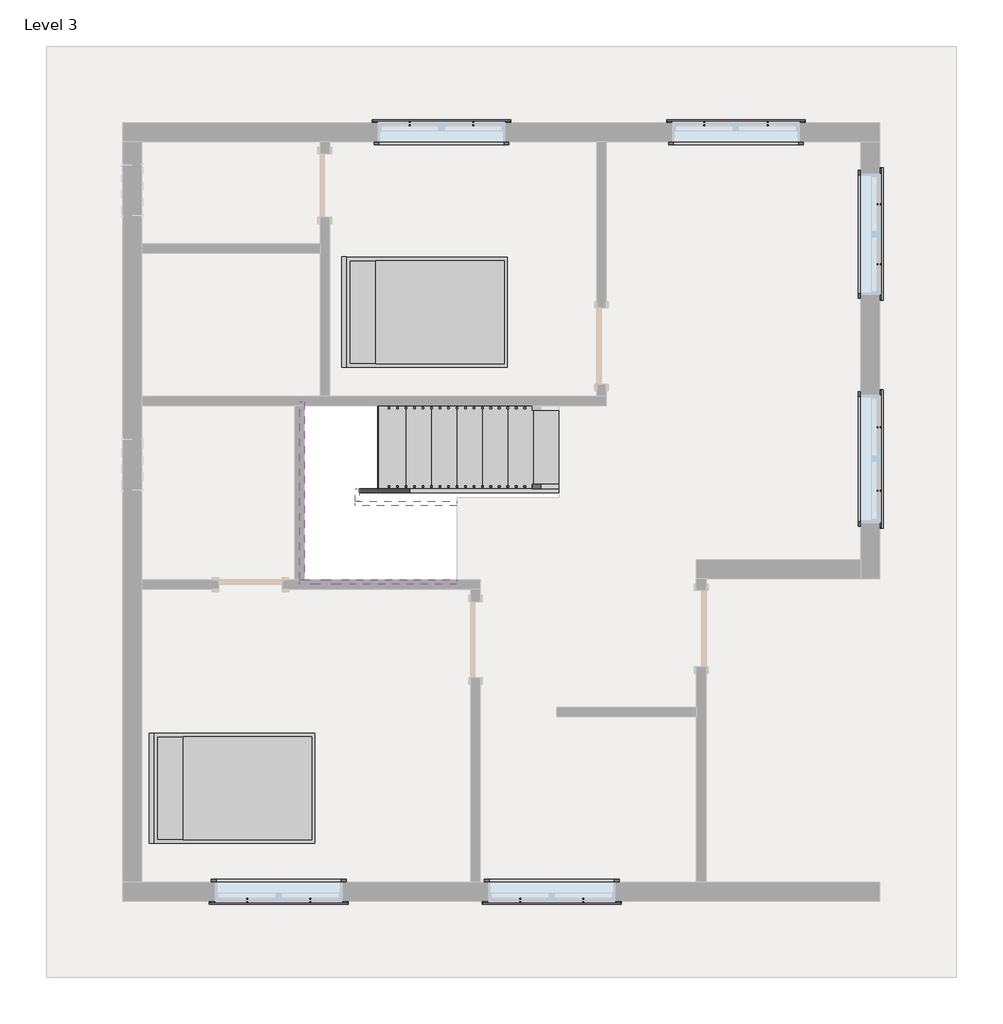
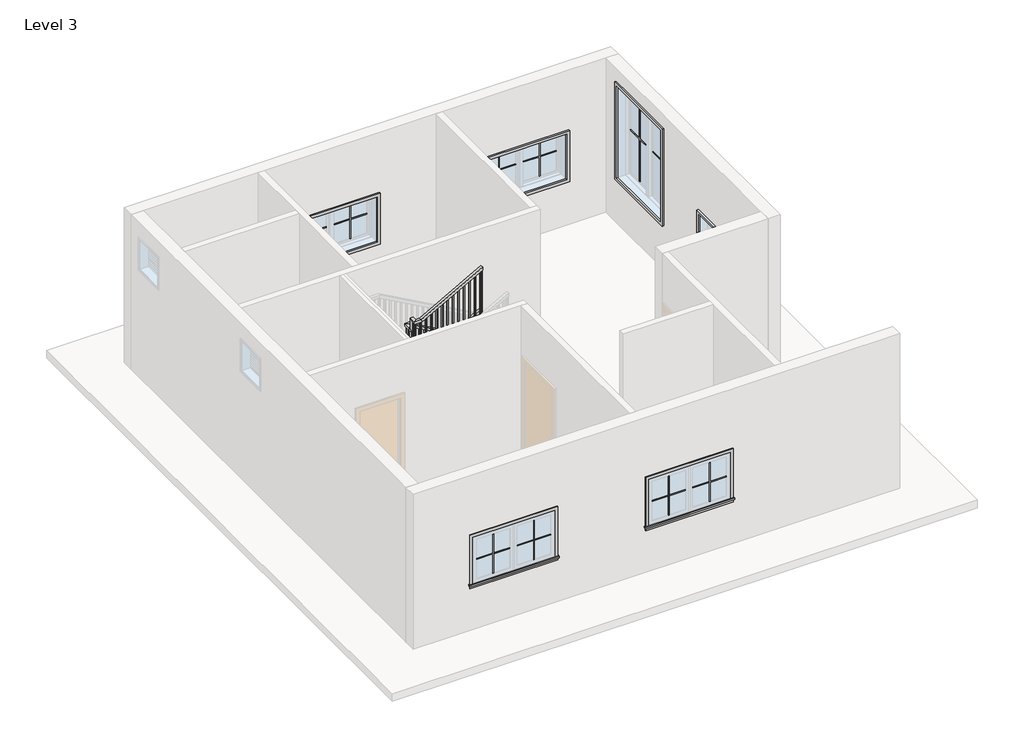
# One storey, part 2 of 2: 24 proxies, 6 members, 2 furniture elements, 1 railing, 1 stair flight.
"""IFC4 building model written with IfcOpenShell, lengths in millimetres."""

from ifc_helpers import new_model, si_unit, frame, origin, place, context, project, spatial, polyline, outline, extrude, faceted_brep, transform, mapped, element, save
from components import muntin_pattern_2x2_muntin_pattern_2x2_9352d081, muntin_pattern_2x2_muntin_pattern_2x2_5c2cbe28, muntin_pattern_2x2_muntin_pattern_2x2_bff912c5, muntin_pattern_2x2_muntin_pattern_2x2_c2194282, trim_window_exterior_flat_with_sill_979bde60, trim_window_exterior_flat_with_sill_e04b3088, trim_window_interior_flat_picture_frame_7883d11b, trim_window_interior_flat_picture_frame_2a7685fe, bed_17739_bed_17739_15c61121, stair_flight_da212e09

model = new_model("IFC4")

# Units and contexts
model_context = context("Model", 3, world=origin())
ifc_project = project(units=[si_unit("LENGTHUNIT", "METRE", prefix="MILLI")], contexts=[model_context])

# Site, building, storey
site = spatial("IfcSite", under=ifc_project)
building = spatial("IfcBuilding", under=site)
storey = spatial("IfcBuildingStorey", under=building, Name="Level 3", Elevation=6248.4)

# Proxies
placement = place(None, origin())
muntin_pattern_2x2_muntin_pattern_2x2_shape = muntin_pattern_2x2_muntin_pattern_2x2_9352d081(model_context)
element("IfcBuildingElementProxy", 1, Name="Muntin Pattern_2x2 : Muntin Pattern_2x2", ObjectType="Muntin Pattern_2x2 : Muntin Pattern_2x2", at=placement, inside=storey, context=model_context, shape_type="MappedRepresentation", body=[
    mapped(muntin_pattern_2x2_muntin_pattern_2x2_shape, transform((-3542.9505704, -5264.0292021, 7232.65), x_axis=(-1.0, 0.0, 0.0), y_axis=(0.0, -1.0, 0.0), z_axis=(0.0, 0.0, 1.0))),
])
element("IfcBuildingElementProxy", 2, Name="Muntin Pattern_2x2 : Muntin Pattern_2x2", ObjectType="Muntin Pattern_2x2 : Muntin Pattern_2x2", at=placement, inside=storey, context=model_context, shape_type="MappedRepresentation", body=[
    mapped(muntin_pattern_2x2_muntin_pattern_2x2_shape, transform((-272.7005704, -5264.0292021, 7232.65), x_axis=(-1.0, 0.0, 0.0), y_axis=(0.0, -1.0, 0.0), z_axis=(0.0, 0.0, 1.0))),
])
element("IfcBuildingElementProxy", 3, Name="Muntin Pattern_2x2 : Muntin Pattern_2x2", ObjectType="Muntin Pattern_2x2 : Muntin Pattern_2x2", at=placement, inside=storey, context=model_context, shape_type="MappedRepresentation", body=[
    mapped(muntin_pattern_2x2_muntin_pattern_2x2_shape, transform((3269.0119296, 401.7582979, 7232.65), x_axis=(0.0, -1.0, 0.0), y_axis=(1.0, 0.0, 0.0), z_axis=(0.0, 0.0, 1.0))),
])
element("IfcBuildingElementProxy", 4, Name="Muntin Pattern_2x2 : Muntin Pattern_2x2", ObjectType="Muntin Pattern_2x2 : Muntin Pattern_2x2", at=placement, inside=storey, context=model_context, shape_type="MappedRepresentation", body=[
    mapped(muntin_pattern_2x2_muntin_pattern_2x2_shape, transform((1175.0994296, 4038.7207979, 7232.65), x_axis=(1.0, 0.0, 0.0), y_axis=(0.0, 1.0, 0.0), z_axis=(0.0, 0.0, 1.0))),
])
element("IfcBuildingElementProxy", 5, Name="Muntin Pattern_2x2 : Muntin Pattern_2x2", ObjectType="Muntin Pattern_2x2 : Muntin Pattern_2x2", at=placement, inside=storey, context=model_context, shape_type="MappedRepresentation", body=[
    mapped(muntin_pattern_2x2_muntin_pattern_2x2_shape, transform((-2352.3255704, 4038.7207979, 7232.65), x_axis=(1.0, 0.0, 0.0), y_axis=(0.0, 1.0, 0.0), z_axis=(0.0, 0.0, 1.0))),
])
muntin_pattern_2x2_muntin_pattern_2x2_2_shape = muntin_pattern_2x2_muntin_pattern_2x2_5c2cbe28(model_context)
element("IfcBuildingElementProxy", 6, Name="Muntin Pattern_2x2 : Muntin Pattern_2x2", ObjectType="Muntin Pattern_2x2 : Muntin Pattern_2x2", at=placement, inside=storey, context=model_context, shape_type="MappedRepresentation", body=[
    mapped(muntin_pattern_2x2_muntin_pattern_2x2_2_shape, transform((-4301.7755704, -5264.0292021, 7232.65), x_axis=(1.0, 0.0, 0.0), y_axis=(0.0, 1.0, 0.0), z_axis=(0.0, 0.0, 1.0))),
])
element("IfcBuildingElementProxy", 7, Name="Muntin Pattern_2x2 : Muntin Pattern_2x2", ObjectType="Muntin Pattern_2x2 : Muntin Pattern_2x2", at=placement, inside=storey, context=model_context, shape_type="MappedRepresentation", body=[
    mapped(muntin_pattern_2x2_muntin_pattern_2x2_2_shape, transform((-1031.5255704, -5264.0292021, 7232.65), x_axis=(1.0, 0.0, 0.0), y_axis=(0.0, 1.0, 0.0), z_axis=(0.0, 0.0, 1.0))),
])
element("IfcBuildingElementProxy", 8, Name="Muntin Pattern_2x2 : Muntin Pattern_2x2", ObjectType="Muntin Pattern_2x2 : Muntin Pattern_2x2", at=placement, inside=storey, context=model_context, shape_type="MappedRepresentation", body=[
    mapped(muntin_pattern_2x2_muntin_pattern_2x2_2_shape, transform((3269.0119296, -357.0667021, 7232.65), x_axis=(0.0, 1.0, 0.0), y_axis=(-1.0, 0.0, 0.0), z_axis=(0.0, 0.0, 1.0))),
])
element("IfcBuildingElementProxy", 9, Name="Muntin Pattern_2x2 : Muntin Pattern_2x2", ObjectType="Muntin Pattern_2x2 : Muntin Pattern_2x2", at=placement, inside=storey, context=model_context, shape_type="MappedRepresentation", body=[
    mapped(muntin_pattern_2x2_muntin_pattern_2x2_2_shape, transform((1933.9244296, 4038.7207979, 7232.65), x_axis=(-1.0, 0.0, 0.0), y_axis=(0.0, -1.0, 0.0), z_axis=(0.0, 0.0, 1.0))),
])
element("IfcBuildingElementProxy", 10, Name="Muntin Pattern_2x2 : Muntin Pattern_2x2", ObjectType="Muntin Pattern_2x2 : Muntin Pattern_2x2", at=placement, inside=storey, context=model_context, shape_type="MappedRepresentation", body=[
    mapped(muntin_pattern_2x2_muntin_pattern_2x2_2_shape, transform((-1593.5005704, 4038.7207979, 7232.65), x_axis=(-1.0, 0.0, 0.0), y_axis=(0.0, -1.0, 0.0), z_axis=(0.0, 0.0, 1.0))),
])
muntin_pattern_2x2_muntin_pattern_2x2_3_shape = muntin_pattern_2x2_muntin_pattern_2x2_bff912c5(model_context)
element("IfcBuildingElementProxy", 11, Name="Muntin Pattern_2x2 : Muntin Pattern_2x2", ObjectType="Muntin Pattern_2x2 : Muntin Pattern_2x2", at=placement, inside=storey, context=model_context, shape_type="MappedRepresentation", body=[
    mapped(muntin_pattern_2x2_muntin_pattern_2x2_3_shape, transform((3269.0119296, 3075.1082979, 7232.65), x_axis=(0.0, -1.0, 0.0), y_axis=(1.0, 0.0, 0.0), z_axis=(0.0, 0.0, 1.0))),
])
muntin_pattern_2x2_muntin_pattern_2x2_4_shape = muntin_pattern_2x2_muntin_pattern_2x2_c2194282(model_context)
element("IfcBuildingElementProxy", 12, Name="Muntin Pattern_2x2 : Muntin Pattern_2x2", ObjectType="Muntin Pattern_2x2 : Muntin Pattern_2x2", at=placement, inside=storey, context=model_context, shape_type="MappedRepresentation", body=[
    mapped(muntin_pattern_2x2_muntin_pattern_2x2_4_shape, transform((3269.0119296, 2354.3832979, 7232.65), x_axis=(0.0, 1.0, 0.0), y_axis=(-1.0, 0.0, 0.0), z_axis=(0.0, 0.0, 1.0))),
])
trim_window_exterior_flat_with_sill_shape = trim_window_exterior_flat_with_sill_979bde60(model_context)
element("IfcBuildingElementProxy", 13, Name="Trim-Window-Exterior-Flat : with Sill", ObjectType="Trim-Window-Exterior-Flat : with Sill", at=placement, inside=storey, context=model_context, shape_type="MappedRepresentation", body=[
    mapped(trim_window_exterior_flat_with_sill_shape, transform((-3922.3630704, -5273.5542021, 8077.2), x_axis=(1.0, 0.0, 0.0), y_axis=(0.0, 0.0, 1.0), z_axis=(0.0, -1.0, 0.0))),
])
element("IfcBuildingElementProxy", 14, Name="Trim-Window-Exterior-Flat : with Sill", ObjectType="Trim-Window-Exterior-Flat : with Sill", at=placement, inside=storey, context=model_context, shape_type="MappedRepresentation", body=[
    mapped(trim_window_exterior_flat_with_sill_shape, transform((-652.1130704, -5273.5542021, 8077.2), x_axis=(1.0, 0.0, 0.0), y_axis=(0.0, 0.0, 1.0), z_axis=(0.0, -1.0, 0.0))),
])
element("IfcBuildingElementProxy", 15, Name="Trim-Window-Exterior-Flat : with Sill", ObjectType="Trim-Window-Exterior-Flat : with Sill", at=placement, inside=storey, context=model_context, shape_type="MappedRepresentation", body=[
    mapped(trim_window_exterior_flat_with_sill_shape, transform((3278.5369296, 22.3457979, 8077.2), x_axis=(0.0, 1.0, 0.0), y_axis=(0.0, 0.0, 1.0), z_axis=(1.0, 0.0, 0.0))),
])
element("IfcBuildingElementProxy", 16, Name="Trim-Window-Exterior-Flat : with Sill", ObjectType="Trim-Window-Exterior-Flat : with Sill", at=placement, inside=storey, context=model_context, shape_type="MappedRepresentation", body=[
    mapped(trim_window_exterior_flat_with_sill_shape, transform((1554.5119296, 4048.2457979, 8077.2), x_axis=(-1.0, 0.0, 0.0), y_axis=(0.0, 0.0, 1.0), z_axis=(0.0, 1.0, 0.0))),
])
element("IfcBuildingElementProxy", 17, Name="Trim-Window-Exterior-Flat : with Sill", ObjectType="Trim-Window-Exterior-Flat : with Sill", at=placement, inside=storey, context=model_context, shape_type="MappedRepresentation", body=[
    mapped(trim_window_exterior_flat_with_sill_shape, transform((-1972.9130704, 4048.2457979, 8077.2), x_axis=(-1.0, 0.0, 0.0), y_axis=(0.0, 0.0, 1.0), z_axis=(0.0, 1.0, 0.0))),
])
trim_window_exterior_flat_with_sill_2_shape = trim_window_exterior_flat_with_sill_e04b3088(model_context)
element("IfcBuildingElementProxy", 18, Name="Trim-Window-Exterior-Flat : with Sill", ObjectType="Trim-Window-Exterior-Flat : with Sill", at=placement, inside=storey, context=model_context, shape_type="MappedRepresentation", body=[
    mapped(trim_window_exterior_flat_with_sill_2_shape, transform((3278.5369296, 2714.7457979, 8991.6), x_axis=(0.0, 1.0, 0.0), y_axis=(0.0, 0.0, 1.0), z_axis=(1.0, 0.0, 0.0))),
])
trim_window_interior_flat_picture_frame_shape = trim_window_interior_flat_picture_frame_7883d11b(model_context)
element("IfcBuildingElementProxy", 19, Name="Trim-Window-Interior-Flat : Picture Frame", ObjectType="Trim-Window-Interior-Flat : Picture Frame", at=placement, inside=storey, context=model_context, shape_type="MappedRepresentation", body=[
    mapped(trim_window_interior_flat_picture_frame_shape, transform((-3922.3630704, -5044.9542021, 8077.2), x_axis=(-1.0, 0.0, 0.0), y_axis=(0.0, 0.0, 1.0), z_axis=(0.0, 1.0, 0.0))),
])
element("IfcBuildingElementProxy", 20, Name="Trim-Window-Interior-Flat : Picture Frame", ObjectType="Trim-Window-Interior-Flat : Picture Frame", at=placement, inside=storey, context=model_context, shape_type="MappedRepresentation", body=[
    mapped(trim_window_interior_flat_picture_frame_shape, transform((-652.1130704, -5044.9542021, 8077.2), x_axis=(-1.0, 0.0, 0.0), y_axis=(0.0, 0.0, 1.0), z_axis=(0.0, 1.0, 0.0))),
])
element("IfcBuildingElementProxy", 21, Name="Trim-Window-Interior-Flat : Picture Frame", ObjectType="Trim-Window-Interior-Flat : Picture Frame", at=placement, inside=storey, context=model_context, shape_type="MappedRepresentation", body=[
    mapped(trim_window_interior_flat_picture_frame_shape, transform((3049.9369296, 22.3457979, 8077.2), x_axis=(0.0, -1.0, 0.0), y_axis=(0.0, 0.0, 1.0), z_axis=(-1.0, 0.0, 0.0))),
])
element("IfcBuildingElementProxy", 22, Name="Trim-Window-Interior-Flat : Picture Frame", ObjectType="Trim-Window-Interior-Flat : Picture Frame", at=placement, inside=storey, context=model_context, shape_type="MappedRepresentation", body=[
    mapped(trim_window_interior_flat_picture_frame_shape, transform((1554.5119296, 3819.6457979, 8077.2), x_axis=(1.0, 0.0, 0.0), y_axis=(0.0, 0.0, 1.0), z_axis=(0.0, -1.0, 0.0))),
])
element("IfcBuildingElementProxy", 23, Name="Trim-Window-Interior-Flat : Picture Frame", ObjectType="Trim-Window-Interior-Flat : Picture Frame", at=placement, inside=storey, context=model_context, shape_type="MappedRepresentation", body=[
    mapped(trim_window_interior_flat_picture_frame_shape, transform((-1972.9130704, 3819.6457979, 8077.2), x_axis=(1.0, 0.0, 0.0), y_axis=(0.0, 0.0, 1.0), z_axis=(0.0, -1.0, 0.0))),
])
trim_window_interior_flat_picture_frame_2_shape = trim_window_interior_flat_picture_frame_2a7685fe(model_context)
element("IfcBuildingElementProxy", 24, Name="Trim-Window-Interior-Flat : Picture Frame", ObjectType="Trim-Window-Interior-Flat : Picture Frame", at=placement, inside=storey, context=model_context, shape_type="MappedRepresentation", body=[
    mapped(trim_window_interior_flat_picture_frame_2_shape, transform((3049.9369296, 2714.7457979, 8991.6), x_axis=(0.0, -1.0, 0.0), y_axis=(0.0, 0.0, 1.0), z_axis=(-1.0, 0.0, 0.0))),
])

# Furniture
bed_17739_bed_17739_shape = bed_17739_bed_17739_15c61121(model_context)
element("IfcFurniture", 25, ObjectType="Bed_17739 : Bed_17739", at=placement, inside=storey, context=model_context, shape_type="MappedRepresentation", body=[
    mapped(bed_17739_bed_17739_shape, transform((-4455.7630704, -3920.5467683, 6248.4), x_axis=(0.0, 1.0, 0.0), y_axis=(-1.0, 0.0, 0.0), z_axis=(0.0, 0.0, 1.0))),
])
element("IfcFurniture", 26, ObjectType="Bed_17739 : Bed_17739", at=placement, inside=storey, context=model_context, shape_type="MappedRepresentation", body=[
    mapped(bed_17739_bed_17739_shape, transform((-2150.7130704, 1781.2957979, 6248.4), x_axis=(0.0, 1.0, 0.0), y_axis=(-1.0, 0.0, 0.0), z_axis=(0.0, 0.0, 1.0))),
])

# Members
element("IfcMember", 27, ObjectType="Stringer - 2\" Width", at=placement, inside=storey, context=model_context, shape_type="SweptSolid", body=[
    extrude(outline(polyline([(6248.4, -569.5630704), (6455.9983948, -569.5630704), (7782.4428392, -2957.1630704), (7433.7641651, -2957.1630704), (6248.4, -823.5075732), (6248.4, -569.5630704)])), frame((0.0, -384.0542021, 0.0), z_axis=(0.0, 1.0, 0.0), x_axis=(0.0, 0.0, 1.0)), (0.0, 0.0, 1.0), 50.8),
])
element("IfcMember", 28, ObjectType="Stringer - 2\" Width", at=placement, inside=storey, context=model_context, shape_type="SweptSolid", body=[
    extrude(outline(polyline([(-3007.9630704, -333.2542021), (-2957.1630704, -333.2542021), (-2957.1630704, -485.6542021), (-3007.9630704, -485.6542021), (-3007.9630704, -333.2542021)])), frame((0.0, 0.0, 7543.8), z_axis=(0.0, 0.0, 1.0), x_axis=(1.0, 0.0, 0.0)), (0.0, 0.0, 1.0), 304.8),
])
element("IfcMember", 29, ObjectType="Stringer - 2\" Width", at=placement, inside=storey, context=model_context, shape_type="SweptSolid", body=[
    extrude(outline(polyline([(7979.9983948, -3007.9630704), (7631.3197207, -3007.9630704), (8308.653054, -1788.7630704), (8657.3317281, -1788.7630704), (7979.9983948, -3007.9630704)])), frame((0.0, -536.4542021, 0.0), z_axis=(0.0, 1.0, 0.0), x_axis=(0.0, 0.0, 1.0)), (0.0, 0.0, 1.0), 50.8),
])
element("IfcMember", 30, ObjectType="Stringer - 2\" Width", at=placement, inside=storey, context=model_context, shape_type="SweptSolid", body=[
    extrude(outline(polyline([(6248.4, -569.5630704), (6455.9983948, -569.5630704), (7848.6, -3076.2459598), (7848.6, -3617.5630704), (7800.653054, -3617.5630704), (6248.4, -823.5075732), (6248.4, -569.5630704)])), frame((0.0, 657.3457979, 0.0), z_axis=(0.0, 1.0, 0.0), x_axis=(0.0, 0.0, 1.0)), (0.0, 0.0, 1.0), 50.8),
])
element("IfcMember", 31, ObjectType="Stringer - 2\" Width", at=placement, inside=storey, context=model_context, shape_type="SweptSolid", body=[
    extrude(outline(polyline([(-3668.3630704, 708.1457979), (-3617.5630704, 708.1457979), (-3617.5630704, -1425.4542021), (-3668.3630704, -1425.4542021), (-3668.3630704, 708.1457979)])), frame((0.0, 0.0, 7543.8), z_axis=(0.0, 0.0, 1.0), x_axis=(1.0, 0.0, 0.0)), (0.0, 0.0, 1.0), 304.8),
])
element("IfcMember", 32, ObjectType="Stringer - 2\" Width", at=placement, inside=storey, context=model_context, shape_type="SweptSolid", body=[
    extrude(outline(polyline([(7613.1095059, -3668.3630704), (7543.8, -3668.3630704), (7543.8, -3165.4985677), (8308.653054, -1788.7630704), (8657.3317281, -1788.7630704), (7613.1095059, -3668.3630704)])), frame((0.0, -1476.2542021, 0.0), z_axis=(0.0, 1.0, 0.0), x_axis=(0.0, 0.0, 1.0)), (0.0, 0.0, 1.0), 50.8),
])

# Railing
element("IfcRailing", 33, ObjectType="Handrail - Rectangular", at=placement, inside=storey, context=model_context, shape_type="SolidModel", body=[
    faceted_brep([(-569.5630704, -333.2542021, 7332.1333333), (-569.5630704, -333.2542021, 7274.020221), (-569.5630704, -282.4542021, 7274.020221), (-569.5630704, -282.4542021, 7332.1333333), (-2931.7630704, -333.2542021, 8644.4666667), (-2982.5630704, -333.2542021, 8614.5757765), (-2982.5630704, -282.4542021, 8614.5757765), (-2931.7630704, -282.4542021, 8644.4666667), (-2931.7630704, -333.2542021, 8686.8), (-2982.5630704, -333.2542021, 8636.0), (-2982.5630704, -282.4542021, 8636.0), (-2931.7630704, -282.4542021, 8686.8), (-3007.9630704, -333.2542021, 8686.8), (-3007.9630704, -333.2542021, 8636.0), (-3058.7630704, -282.4542021, 8636.0), (-3058.7630704, -282.4542021, 8686.8), (-3007.9630704, -409.4542021, 8686.8), (-3007.9630704, -409.4542021, 8636.0), (-3058.7630704, -409.4542021, 8636.0), (-3058.7630704, -409.4542021, 8686.8), (-3007.9630704, -460.2542021, 8686.8), (-3007.9630704, -511.0542021, 8636.0), (-3058.7630704, -511.0542021, 8636.0), (-3058.7630704, -460.2542021, 8686.8), (-3007.9630704, -460.2542021, 8898.4666667), (-3007.9630704, -511.0542021, 8847.6666667), (-3058.7630704, -511.0542021, 8847.6666667), (-3058.7630704, -460.2542021, 8898.4666667), (-3007.9630704, -536.4542021, 8898.4666667), (-3007.9630704, -536.4542021, 8847.6666667), (-3058.7630704, -587.2542021, 8847.6666667), (-3058.7630704, -587.2542021, 8898.4666667), (-2931.7630704, -536.4542021, 8898.4666667), (-2918.5994682, -536.4542021, 8847.6666667), (-2918.5994682, -587.2542021, 8847.6666667), (-2931.7630704, -587.2542021, 8898.4666667), (-1788.7630704, -536.4542021, 9533.4666667), (-1788.7630704, -587.2542021, 9533.4666667), (-1788.7630704, -587.2542021, 9475.3535543), (-1788.7630704, -536.4542021, 9475.3535543)], [[[0, 1, 2, 3]], [[1, 0, 4, 5]], [[2, 1, 5, 6]], [[3, 2, 6, 7]], [[0, 3, 7, 4]], [[5, 4, 8, 9]], [[6, 5, 9, 10]], [[7, 6, 10, 11]], [[4, 7, 11, 8]], [[9, 8, 12, 13]], [[10, 9, 13, 14]], [[11, 10, 14, 15]], [[8, 11, 15, 12]], [[13, 12, 16, 17]], [[14, 13, 17, 18]], [[15, 14, 18, 19]], [[12, 15, 19, 16]], [[17, 16, 20, 21]], [[18, 17, 21, 22]], [[19, 18, 22, 23]], [[16, 19, 23, 20]], [[21, 20, 24, 25]], [[22, 21, 25, 26]], [[23, 22, 26, 27]], [[20, 23, 27, 24]], [[25, 24, 28, 29]], [[26, 25, 29, 30]], [[27, 26, 30, 31]], [[24, 27, 31, 28]], [[29, 28, 32, 33]], [[30, 29, 33, 34]], [[31, 30, 34, 35]], [[28, 31, 35, 32]], [[36, 37, 38, 39]], [[33, 32, 36, 39]], [[34, 33, 39, 38]], [[35, 34, 38, 37]], [[32, 35, 37, 36]]]),
    extrude(outline(polyline([(9455.9507765, -1823.6880704), (8449.7333333, -1823.6880704), (8449.7333333, -1804.6380704), (9466.5341099, -1804.6380704), (9455.9507765, -1823.6880704)])), frame((0.0, -571.3792021, 0.0), z_axis=(0.0, 1.0, 0.0), x_axis=(0.0, 0.0, 1.0)), (0.0, 0.0, 1.0), 19.05),
    extrude(outline(polyline([(9399.5063321, -1925.2880704), (8449.7333333, -1925.2880704), (8449.7333333, -1906.2380704), (9410.0896654, -1906.2380704), (9399.5063321, -1925.2880704)])), frame((0.0, -571.3792021, 0.0), z_axis=(0.0, 1.0, 0.0), x_axis=(0.0, 0.0, 1.0)), (0.0, 0.0, 1.0), 19.05),
    extrude(outline(polyline([(9343.0618876, -2026.8880704), (8449.7333333, -2026.8880704), (8449.7333333, -2007.8380704), (9353.645221, -2007.8380704), (9343.0618876, -2026.8880704)])), frame((0.0, -571.3792021, 0.0), z_axis=(0.0, 1.0, 0.0), x_axis=(0.0, 0.0, 1.0)), (0.0, 0.0, 1.0), 19.05),
    extrude(outline(polyline([(9286.6174432, -2128.4880704), (8280.4, -2128.4880704), (8280.4, -2109.4380704), (9297.2007765, -2109.4380704), (9286.6174432, -2128.4880704)])), frame((0.0, -571.3792021, 0.0), z_axis=(0.0, 1.0, 0.0), x_axis=(0.0, 0.0, 1.0)), (0.0, 0.0, 1.0), 19.05),
    extrude(outline(polyline([(9230.1729988, -2230.0880704), (8280.4, -2230.0880704), (8280.4, -2211.0380704), (9240.7563321, -2211.0380704), (9230.1729988, -2230.0880704)])), frame((0.0, -571.3792021, 0.0), z_axis=(0.0, 1.0, 0.0), x_axis=(0.0, 0.0, 1.0)), (0.0, 0.0, 1.0), 19.05),
    extrude(outline(polyline([(9173.7285543, -2331.6880704), (8280.4, -2331.6880704), (8280.4, -2312.6380704), (9184.3118876, -2312.6380704), (9173.7285543, -2331.6880704)])), frame((0.0, -571.3792021, 0.0), z_axis=(0.0, 1.0, 0.0), x_axis=(0.0, 0.0, 1.0)), (0.0, 0.0, 1.0), 19.05),
    extrude(outline(polyline([(9117.2841099, -2433.2880704), (8111.0666667, -2433.2880704), (8111.0666667, -2414.2380704), (9127.8674432, -2414.2380704), (9117.2841099, -2433.2880704)])), frame((0.0, -571.3792021, 0.0), z_axis=(0.0, 1.0, 0.0), x_axis=(0.0, 0.0, 1.0)), (0.0, 0.0, 1.0), 19.05),
    extrude(outline(polyline([(9060.8396654, -2534.8880704), (8111.0666667, -2534.8880704), (8111.0666667, -2515.8380704), (9071.4229988, -2515.8380704), (9060.8396654, -2534.8880704)])), frame((0.0, -571.3792021, 0.0), z_axis=(0.0, 1.0, 0.0), x_axis=(0.0, 0.0, 1.0)), (0.0, 0.0, 1.0), 19.05),
    extrude(outline(polyline([(9004.395221, -2636.4880704), (8111.0666667, -2636.4880704), (8111.0666667, -2617.4380704), (9014.9785543, -2617.4380704), (9004.395221, -2636.4880704)])), frame((0.0, -571.3792021, 0.0), z_axis=(0.0, 1.0, 0.0), x_axis=(0.0, 0.0, 1.0)), (0.0, 0.0, 1.0), 19.05),
    extrude(outline(polyline([(8947.9507765, -2738.0880704), (7941.7333333, -2738.0880704), (7941.7333333, -2719.0380704), (8958.5341099, -2719.0380704), (8947.9507765, -2738.0880704)])), frame((0.0, -571.3792021, 0.0), z_axis=(0.0, 1.0, 0.0), x_axis=(0.0, 0.0, 1.0)), (0.0, 0.0, 1.0), 19.05),
    extrude(outline(polyline([(8891.5063321, -2839.6880704), (7941.7333333, -2839.6880704), (7941.7333333, -2820.6380704), (8902.0896654, -2820.6380704), (8891.5063321, -2839.6880704)])), frame((0.0, -571.3792021, 0.0), z_axis=(0.0, 1.0, 0.0), x_axis=(0.0, 0.0, 1.0)), (0.0, 0.0, 1.0), 19.05),
    extrude(outline(polyline([(8835.0618876, -2941.2880704), (7941.7333333, -2941.2880704), (7941.7333333, -2922.2380704), (8845.645221, -2922.2380704), (8835.0618876, -2941.2880704)])), frame((0.0, -571.3792021, 0.0), z_axis=(0.0, 1.0, 0.0), x_axis=(0.0, 0.0, 1.0)), (0.0, 0.0, 1.0), 19.05),
    extrude(outline(polyline([(-3023.8380704, -501.5292021), (-3023.8380704, -520.5792021), (-3042.8880704, -520.5792021), (-3042.8880704, -501.5292021), (-3023.8380704, -501.5292021)])), frame((0.0, 0.0, 7772.4), z_axis=(0.0, 0.0, 1.0), x_axis=(1.0, 0.0, 0.0)), (0.0, 0.0, 1.0), 1075.2666667),
    extrude(outline(polyline([(-3023.8380704, -399.9292021), (-3023.8380704, -418.9792021), (-3042.8880704, -418.9792021), (-3042.8880704, -399.9292021), (-3023.8380704, -399.9292021)])), frame((0.0, 0.0, 7772.4), z_axis=(0.0, 0.0, 1.0), x_axis=(1.0, 0.0, 0.0)), (0.0, 0.0, 1.0), 863.6),
    extrude(outline(polyline([(-2998.4380704, -317.3792021), (-3017.4880704, -317.3792021), (-3017.4880704, -298.3292021), (-2998.4380704, -298.3292021), (-2998.4380704, -317.3792021)])), frame((0.0, 0.0, 7772.4), z_axis=(0.0, 0.0, 1.0), x_axis=(1.0, 0.0, 0.0)), (0.0, 0.0, 1.0), 863.6),
    extrude(outline(polyline([(8577.5341099, -2915.8880704), (7603.0666667, -2915.8880704), (7603.0666667, -2896.8380704), (8566.9507765, -2896.8380704), (8577.5341099, -2915.8880704)])), frame((0.0, -317.3792021, 0.0), z_axis=(0.0, 1.0, 0.0), x_axis=(0.0, 0.0, 1.0)), (0.0, 0.0, 1.0), 19.05),
    extrude(outline(polyline([(8521.0896654, -2814.2880704), (7603.0666667, -2814.2880704), (7603.0666667, -2795.2380704), (8510.5063321, -2795.2380704), (8521.0896654, -2814.2880704)])), frame((0.0, -317.3792021, 0.0), z_axis=(0.0, 1.0, 0.0), x_axis=(0.0, 0.0, 1.0)), (0.0, 0.0, 1.0), 19.05),
    extrude(outline(polyline([(8464.645221, -2712.6880704), (7603.0666667, -2712.6880704), (7603.0666667, -2693.6380704), (8454.0618876, -2693.6380704), (8464.645221, -2712.6880704)])), frame((0.0, -317.3792021, 0.0), z_axis=(0.0, 1.0, 0.0), x_axis=(0.0, 0.0, 1.0)), (0.0, 0.0, 1.0), 19.05),
    extrude(outline(polyline([(8408.2007765, -2611.0880704), (7433.7333333, -2611.0880704), (7433.7333333, -2592.0380704), (8397.6174432, -2592.0380704), (8408.2007765, -2611.0880704)])), frame((0.0, -317.3792021, 0.0), z_axis=(0.0, 1.0, 0.0), x_axis=(0.0, 0.0, 1.0)), (0.0, 0.0, 1.0), 19.05),
    extrude(outline(polyline([(8351.7563321, -2509.4880704), (7433.7333333, -2509.4880704), (7433.7333333, -2490.4380704), (8341.1729988, -2490.4380704), (8351.7563321, -2509.4880704)])), frame((0.0, -317.3792021, 0.0), z_axis=(0.0, 1.0, 0.0), x_axis=(0.0, 0.0, 1.0)), (0.0, 0.0, 1.0), 19.05),
    extrude(outline(polyline([(8295.3118876, -2407.8880704), (7433.7333333, -2407.8880704), (7433.7333333, -2388.8380704), (8284.7285543, -2388.8380704), (8295.3118876, -2407.8880704)])), frame((0.0, -317.3792021, 0.0), z_axis=(0.0, 1.0, 0.0), x_axis=(0.0, 0.0, 1.0)), (0.0, 0.0, 1.0), 19.05),
    extrude(outline(polyline([(8238.8674432, -2306.2880704), (7264.4, -2306.2880704), (7264.4, -2287.2380704), (8228.2841099, -2287.2380704), (8238.8674432, -2306.2880704)])), frame((0.0, -317.3792021, 0.0), z_axis=(0.0, 1.0, 0.0), x_axis=(0.0, 0.0, 1.0)), (0.0, 0.0, 1.0), 19.05),
    extrude(outline(polyline([(8182.4229988, -2204.6880704), (7264.4, -2204.6880704), (7264.4, -2185.6380704), (8171.8396654, -2185.6380704), (8182.4229988, -2204.6880704)])), frame((0.0, -317.3792021, 0.0), z_axis=(0.0, 1.0, 0.0), x_axis=(0.0, 0.0, 1.0)), (0.0, 0.0, 1.0), 19.05),
    extrude(outline(polyline([(8125.9785543, -2103.0880704), (7264.4, -2103.0880704), (7264.4, -2084.0380704), (8115.395221, -2084.0380704), (8125.9785543, -2103.0880704)])), frame((0.0, -317.3792021, 0.0), z_axis=(0.0, 1.0, 0.0), x_axis=(0.0, 0.0, 1.0)), (0.0, 0.0, 1.0), 19.05),
    extrude(outline(polyline([(8069.5341099, -2001.4880704), (7095.0666667, -2001.4880704), (7095.0666667, -1982.4380704), (8058.9507765, -1982.4380704), (8069.5341099, -2001.4880704)])), frame((0.0, -317.3792021, 0.0), z_axis=(0.0, 1.0, 0.0), x_axis=(0.0, 0.0, 1.0)), (0.0, 0.0, 1.0), 19.05),
    extrude(outline(polyline([(8013.0896654, -1899.8880704), (7095.0666667, -1899.8880704), (7095.0666667, -1880.8380704), (8002.5063321, -1880.8380704), (8013.0896654, -1899.8880704)])), frame((0.0, -317.3792021, 0.0), z_axis=(0.0, 1.0, 0.0), x_axis=(0.0, 0.0, 1.0)), (0.0, 0.0, 1.0), 19.05),
    extrude(outline(polyline([(7956.645221, -1798.2880704), (7095.0666667, -1798.2880704), (7095.0666667, -1779.2380704), (7946.0618876, -1779.2380704), (7956.645221, -1798.2880704)])), frame((0.0, -317.3792021, 0.0), z_axis=(0.0, 1.0, 0.0), x_axis=(0.0, 0.0, 1.0)), (0.0, 0.0, 1.0), 19.05),
    extrude(outline(polyline([(7900.2007765, -1696.6880704), (6925.7333333, -1696.6880704), (6925.7333333, -1677.6380704), (7889.6174432, -1677.6380704), (7900.2007765, -1696.6880704)])), frame((0.0, -317.3792021, 0.0), z_axis=(0.0, 1.0, 0.0), x_axis=(0.0, 0.0, 1.0)), (0.0, 0.0, 1.0), 19.05),
    extrude(outline(polyline([(7843.7563321, -1595.0880704), (6925.7333333, -1595.0880704), (6925.7333333, -1576.0380704), (7833.1729988, -1576.0380704), (7843.7563321, -1595.0880704)])), frame((0.0, -317.3792021, 0.0), z_axis=(0.0, 1.0, 0.0), x_axis=(0.0, 0.0, 1.0)), (0.0, 0.0, 1.0), 19.05),
    extrude(outline(polyline([(7787.3118876, -1493.4880704), (6925.7333333, -1493.4880704), (6925.7333333, -1474.4380704), (7776.7285543, -1474.4380704), (7787.3118876, -1493.4880704)])), frame((0.0, -317.3792021, 0.0), z_axis=(0.0, 1.0, 0.0), x_axis=(0.0, 0.0, 1.0)), (0.0, 0.0, 1.0), 19.05),
    extrude(outline(polyline([(7730.8674432, -1391.8880704), (6756.4, -1391.8880704), (6756.4, -1372.8380704), (7720.2841099, -1372.8380704), (7730.8674432, -1391.8880704)])), frame((0.0, -317.3792021, 0.0), z_axis=(0.0, 1.0, 0.0), x_axis=(0.0, 0.0, 1.0)), (0.0, 0.0, 1.0), 19.05),
    extrude(outline(polyline([(7674.4229988, -1290.2880704), (6756.4, -1290.2880704), (6756.4, -1271.2380704), (7663.8396654, -1271.2380704), (7674.4229988, -1290.2880704)])), frame((0.0, -317.3792021, 0.0), z_axis=(0.0, 1.0, 0.0), x_axis=(0.0, 0.0, 1.0)), (0.0, 0.0, 1.0), 19.05),
    extrude(outline(polyline([(7617.9785543, -1188.6880704), (6756.4, -1188.6880704), (6756.4, -1169.6380704), (7607.395221, -1169.6380704), (7617.9785543, -1188.6880704)])), frame((0.0, -317.3792021, 0.0), z_axis=(0.0, 1.0, 0.0), x_axis=(0.0, 0.0, 1.0)), (0.0, 0.0, 1.0), 19.05),
    extrude(outline(polyline([(7561.5341099, -1087.0880704), (6587.0666667, -1087.0880704), (6587.0666667, -1068.0380704), (7550.9507765, -1068.0380704), (7561.5341099, -1087.0880704)])), frame((0.0, -317.3792021, 0.0), z_axis=(0.0, 1.0, 0.0), x_axis=(0.0, 0.0, 1.0)), (0.0, 0.0, 1.0), 19.05),
    extrude(outline(polyline([(7505.0896654, -985.4880704), (6587.0666667, -985.4880704), (6587.0666667, -966.4380704), (7494.5063321, -966.4380704), (7505.0896654, -985.4880704)])), frame((0.0, -317.3792021, 0.0), z_axis=(0.0, 1.0, 0.0), x_axis=(0.0, 0.0, 1.0)), (0.0, 0.0, 1.0), 19.05),
    extrude(outline(polyline([(7448.645221, -883.8880704), (6587.0666667, -883.8880704), (6587.0666667, -864.8380704), (7438.0618876, -864.8380704), (7448.645221, -883.8880704)])), frame((0.0, -317.3792021, 0.0), z_axis=(0.0, 1.0, 0.0), x_axis=(0.0, 0.0, 1.0)), (0.0, 0.0, 1.0), 19.05),
    extrude(outline(polyline([(7392.2007765, -782.2880704), (6417.7333333, -782.2880704), (6417.7333333, -763.2380704), (7381.6174432, -763.2380704), (7392.2007765, -782.2880704)])), frame((0.0, -317.3792021, 0.0), z_axis=(0.0, 1.0, 0.0), x_axis=(0.0, 0.0, 1.0)), (0.0, 0.0, 1.0), 19.05),
    extrude(outline(polyline([(7335.7563321, -680.6880704), (6417.7333333, -680.6880704), (6417.7333333, -661.6380704), (7325.1729988, -661.6380704), (7335.7563321, -680.6880704)])), frame((0.0, -317.3792021, 0.0), z_axis=(0.0, 1.0, 0.0), x_axis=(0.0, 0.0, 1.0)), (0.0, 0.0, 1.0), 19.05),
    extrude(outline(polyline([(-3023.8380704, -552.3292021), (-3023.8380704, -571.3792021), (-3042.8880704, -571.3792021), (-3042.8880704, -552.3292021), (-3023.8380704, -552.3292021)])), frame((0.0, 0.0, 7772.4), z_axis=(0.0, 0.0, 1.0), x_axis=(1.0, 0.0, 0.0)), (0.0, 0.0, 1.0), 1075.2666667),
    extrude(outline(polyline([(-3023.8380704, -317.3792021), (-3042.8880704, -317.3792021), (-3042.8880704, -298.3292021), (-3023.8380704, -298.3292021), (-3023.8380704, -317.3792021)])), frame((0.0, 0.0, 7772.4), z_axis=(0.0, 0.0, 1.0), x_axis=(1.0, 0.0, 0.0)), (0.0, 0.0, 1.0), 863.6),
    extrude(outline(polyline([(9464.770221, -1807.8130704), (8449.7333333, -1807.8130704), (8449.7333333, -1788.7630704), (9475.3535543, -1788.7630704), (9464.770221, -1807.8130704)])), frame((0.0, -571.3792021, 0.0), z_axis=(0.0, 1.0, 0.0), x_axis=(0.0, 0.0, 1.0)), (0.0, 0.0, 1.0), 19.05),
    extrude(outline(polyline([(7284.6035543, -588.6130704), (6417.7333333, -588.6130704), (6417.7333333, -569.5630704), (7274.020221, -569.5630704), (7284.6035543, -588.6130704)])), frame((0.0, -317.3792021, 0.0), z_axis=(0.0, 1.0, 0.0), x_axis=(0.0, 0.0, 1.0)), (0.0, 0.0, 1.0), 19.05),
])

# Stair flight
stair_flight_shape = stair_flight_da212e09(model_context)
element("IfcStairFlight", 34, ObjectType="2\" Tread 1\" Nosing 1/4\" Riser", at=placement, inside=storey, context=model_context, shape_type="MappedRepresentation", body=[
    mapped(stair_flight_shape, transform((0.0, 0.0, 0.0), x_axis=(1.0, 0.0, 0.0), y_axis=(0.0, 1.0, 0.0), z_axis=(0.0, 0.0, 1.0))),
])

save(model, "model.ifc")

# Revit data of these elements
# Type "Muntin Pattern_2x2 : Muntin Pattern_2x2"
#   Width [instance default] = 4' - 0"
#   Thickness = 0' - 0 1/2"
#   Height [instance default] = 4' - 0"
#   Distance = 0' - 0 3/4"
#   Interior Material [instance default] = none
#   Exterior Material [instance default] = none
#   Default Elevation = 0
# Type "Trim-Window-Exterior-Flat : with Sill"
#   Trim Width = 0' - 2 1/4"
#   Trim Thickness_Picture Frame = 0' - 1 1/4"
#   Trim Thickness_with Sill = 0' - 0 3/4"
#   Sill Thickness = 0' - 1 1/4"
#   Opening Width [instance default] = 2' - 0"
#   Opening Height [instance default] = 3' - 0"
#   Default Elevation = 4' - 0"
#   Sill = yes
#   Picture Frame = no
#   Trim Material [instance default] = none
# Type "Trim-Window-Interior-Flat : Picture Frame"
#   Trim Thickness_Picture Frame = 0' - 1 1/4"
#   Trim Width = 0' - 2 1/4"
#   Trim Thickness_with Sill = 0' - 0 3/4"
#   Sill Thickness = 0' - 1 1/4"
#   Opening Width [instance default] = 2' - 0"
#   Opening Height [instance default] = 3' - 0"
#   Default Elevation = 4' - 0"
#   Sill = no
#   Picture Frame = yes
#   Trim Material [instance default] = none
# Type "Bed_17739 : Bed_17739"
#   Default Elevation = 0
# Type "Handrail - Rectangular"
#   Assembly Code = "C2010400"
#   built-in parameter 1008612 = 0.0416667 (stored number, unit not read)
#   built-in parameter 1008611 = 0.0416667 (stored number, unit not read)
#   built-in parameter 1008609 = 0.333333 (stored number, unit not read)
#   built-in parameter 1008604 = 0.166667 (stored number, unit not read)
#   built-in parameter 1008603 = 0.166667 (stored number, unit not read)
#   Railing Height = 3' - 0"
#   built-in parameter 1008630 = 2
#   built-in parameter 1008610 = 2
#   built-in parameter 1008618 = Baluster - Square : 3/4"
# Elements 1, 2, 3, 4, 5, 6, 7, 8, 9, 10 (IfcBuildingElementProxy, "Muntin Pattern_2x2 : Muntin Pattern_2x2")
#   Width = 2' - 0 5/8"
#   Height = 2' - 6 1/2"
#   Interior Material = Wood - Stained
#   Exterior Material = Clad - White
#   Phase Created = New Construction
#   Materials on its faces: "Clad - White", "Wood - Stained"
# Elements 11, 12 (IfcBuildingElementProxy, "Muntin Pattern_2x2 : Muntin Pattern_2x2")
#   Width = 1' - 11 1/8"
#   Height = 5' - 6 1/2"
#   Interior Material = Wood - Stained
#   Exterior Material = Clad - White
#   Phase Created = New Construction
#   Materials on its faces: "Clad - White", "Wood - Stained"
# Elements 13, 14, 15, 16, 17 (IfcBuildingElementProxy, "Trim-Window-Exterior-Flat : with Sill")
#   Opening Width = 5' - 0"
#   Opening Height = 3' - 0"
#   Trim Material = Clad - White
#   Phase Created = New Construction
#   Materials on its faces: "Clad - White"
# Element 18 (IfcBuildingElementProxy, "Trim-Window-Exterior-Flat : with Sill")
#   Opening Width = 4' - 9"
#   Opening Height = 6' - 0"
#   Trim Material = Clad - White
#   Phase Created = New Construction
#   Materials on its faces: "Clad - White"
# Elements 19, 20, 21, 22, 23 (IfcBuildingElementProxy, "Trim-Window-Interior-Flat : Picture Frame")
#   Opening Width = 5' - 0"
#   Opening Height = 3' - 0"
#   Trim Material = Wood - Stained
#   Phase Created = New Construction
#   Materials on its faces: "Wood - Stained"
# Element 24 (IfcBuildingElementProxy, "Trim-Window-Interior-Flat : Picture Frame")
#   Opening Width = 4' - 9"
#   Opening Height = 6' - 0"
#   Trim Material = Wood - Stained
#   Phase Created = New Construction
#   Materials on its faces: "Wood - Stained"
# Elements 25, 26 (IfcFurniture, "Bed_17739 : Bed_17739")
#   Phase Created = New Construction
#   Materials on its faces: "legs", "sheets", "bed frame", "Blanket"
# Elements 27, 28, 29, 30, 31, 32 (IfcMember, "Stringer - 2\" Width")
#   Phase Created = New Construction
# Element 33 (IfcRailing, "Handrail - Rectangular")
#   Phase Created = New Construction
# Element 34 (IfcStairFlight, "2\" Tread 1\" Nosing 1/4\" Riser")
#   Phase Created = New Construction
# Materials
#   "Clad - White": class "Wood", colour RGB 242 242 238, transparency 0, Cost = 0
#   "Wood - Stained": class "Wood", colour RGB 224 178 126, transparency 0, Cost = 0
#   "legs": colour RGB 90 73 37, transparency 0, Cost = 0
#   "sheets": colour RGB 200 195 176, transparency 0, Cost = 0
#   "bed frame": colour RGB 90 73 37, transparency 0, Cost = 0
#   "Blanket": class "System", colour RGB 59 0 1, transparency 0, Cost = 0
